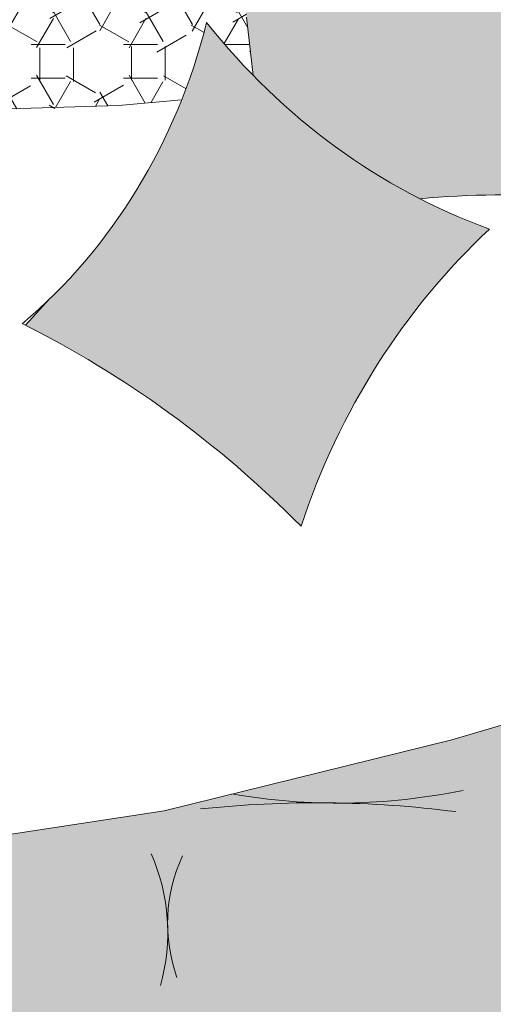
# Model space of a CAD drawing. Units: inches. Extents: x 1994 to 3075, y 3517 to 3950.
# Tile 43 of 58: x 1994.65094 to 1994.66748, y 3553.72103 to 3553.75542. Entities that reach past the tile are written whole.
import ezdxf

# ---------------------------------------------------------------- set-up
doc = ezdxf.new("R2010")
doc.units = ezdxf.units.IN
doc.layers.add('A-FURN-REFR', color=8, linetype='Continuous', lineweight=13)
doc.layers.add('A-FURN-REFR-PATT', color=8, linetype='Continuous', lineweight=13)

msp = doc.modelspace()

# ---------------------------------------------------------------- hatches: boundary and pattern name
at = {"layer": 'A-FURN-REFR-PATT'}
h = msp.add_hatch(dxfattribs=at)
h.set_pattern_fill('ESA_QT1', color=256, scale=0.001181, style=0, pattern_type=2)
h.set_pattern_definition([(0, (2000.7131367, 3549.95567), (0.0016133858, 0.0027944882), [0.0011811024, -0.0020457874]), (0, (2000.7131367, 3549.956851), (0.0016133858, 0.0027944882), [0.0011811024, -0.0020457874]), (60, (2000.7147507, 3549.9540566), (-0.0016134048, 0.0027944772), [0.0011811024, -0.0020457874]), (60, (2000.7137272, 3549.9546472), (-0.0016134048, 0.0027944772), [0.0011811024, -0.0020457874]), (120, (2000.7159311, 3549.9540566), (-0.0032267907, -1.1e-08), [0.0011811024, -0.0020457874]), (120, (2000.716954, 3549.9546472), (-0.0032267907, -1.1e-08), [0.0011811024, -0.0020457874]), (90, (2000.7131367, 3549.95567), (-0.00161338583, 0.0027944882), [0.0011811024, -0.0044079921]), (90, (2000.7143178, 3549.95567), (-0.00161338583, 0.0027944882), [0.0011811024, -0.0044079921]), (30, (2000.7159311, 3549.9540566), (0.00161340485, 0.0027944772), [0.0011811024, -0.0044079921]), (150, (2000.71475, 3549.9540566), (-0.00322679068, 1.1e-08), [0.0011811024, -0.0044079921]), (30, (2000.7153406, 3549.9550795), (0.00161340485, 0.0027944772), [0.0011811024, -0.0044079921]), (150, (2000.7153406, 3549.9550795), (-0.00322679068, 1.1e-08), [0.0011811024, -0.0044079921])])
edge = h.paths.add_edge_path()
edge.add_ellipse((1994.640876, 3553.752584), major_axis=(0, 0.019971), ratio=0.910403, start_angle=279.2385, end_angle=295.7126)
edge.add_ellipse((1994.661382, 3553.784799), major_axis=(0, 0.024564), ratio=0.910403, start_angle=170.9484, end_angle=180.8636)
edge.add_line((1994.661753, 3553.760238), (1994.660448, 3553.761168))
edge.add_line((1994.660448, 3553.761168), (1994.657839, 3553.762473))
edge.add_line((1994.657839, 3553.762473), (1994.656621, 3553.763504))
edge.add_line((1994.656621, 3553.763504), (1994.655861, 3553.763272))
edge.add_line((1994.655861, 3553.763272), (1994.655293, 3553.763476))
edge.add_line((1994.655293, 3553.763476), (1994.655493, 3553.762522))
edge.add_line((1994.655493, 3553.762522), (1994.655292, 3553.760584))
edge.add_line((1994.655292, 3553.760584), (1994.655292, 3553.760424))
edge.add_line((1994.655292, 3553.760424), (1994.655994, 3553.759788))
edge.add_line((1994.655994, 3553.759788), (1994.656079, 3553.758256))
edge.add_line((1994.656079, 3553.758256), (1994.654831, 3553.75802))
edge.add_line((1994.654831, 3553.75802), (1994.653607, 3553.75863))
edge.add_line((1994.653607, 3553.75863), (1994.651194, 3553.757931))
edge.add_line((1994.651194, 3553.757931), (1994.647697, 3553.757851))
edge.add_line((1994.647697, 3553.757851), (1994.645839, 3553.758008))
edge.add_line((1994.645839, 3553.758008), (1994.644836, 3553.757661))
edge.add_line((1994.644836, 3553.757661), (1994.64177, 3553.757379))
edge.add_line((1994.64177, 3553.757379), (1994.63952, 3553.757537))
edge.add_line((1994.63952, 3553.757537), (1994.636664, 3553.757269))
edge.add_line((1994.636664, 3553.757269), (1994.635142, 3553.757511))
edge.add_line((1994.635142, 3553.757511), (1994.634583, 3553.7569))
edge.add_line((1994.634583, 3553.7569), (1994.633061, 3553.756568))
edge.add_line((1994.633061, 3553.756568), (1994.631936, 3553.756647))
edge.add_line((1994.631936, 3553.756647), (1994.631946, 3553.757723))
edge.add_line((1994.631946, 3553.757723), (1994.632293, 3553.759053))
edge.add_line((1994.632293, 3553.759053), (1994.631942, 3553.760336))
edge.add_line((1994.631942, 3553.760336), (1994.631857, 3553.761868))
edge.add_line((1994.631857, 3553.761868), (1994.63213, 3553.76327))
edge.add_line((1994.63213, 3553.76327), (1994.632168, 3553.765117))
edge.add_line((1994.632168, 3553.765117), (1994.631874, 3553.766635))
edge.add_line((1994.631874, 3553.766635), (1994.632212, 3553.768118))
edge.add_line((1994.632212, 3553.768118), (1994.631521, 3553.769225))
edge.add_line((1994.631521, 3553.769225), (1994.631256, 3553.770206))
edge.add_line((1994.631256, 3553.770206), (1994.631719, 3553.770698))
edge.add_line((1994.631719, 3553.770698), (1994.632688, 3553.770917))
edge.add_line((1994.632688, 3553.770917), (1994.633747, 3553.770757))
edge.add_line((1994.633747, 3553.770757), (1994.63499, 3553.77107))
edge.add_line((1994.63499, 3553.77107), (1994.637864, 3553.771031))
edge.add_line((1994.637864, 3553.771031), (1994.638857, 3553.770678))
edge.add_line((1994.638857, 3553.770678), (1994.641165, 3553.770867))
edge.add_line((1994.641165, 3553.770867), (1994.645224, 3553.770907))
edge.add_line((1994.645224, 3553.770907), (1994.645865, 3553.770719))
edge.add_line((1994.645865, 3553.770719), (1994.647785, 3553.771462))
edge.add_line((1994.647785, 3553.771462), (1994.650215, 3553.771855))
edge.add_line((1994.650215, 3553.771855), (1994.65289, 3553.771785))
edge.add_line((1994.65289, 3553.771785), (1994.653416, 3553.772222))
edge.add_line((1994.653416, 3553.772222), (1994.654716, 3553.77277))
edge.add_line((1994.654716, 3553.77277), (1994.655776, 3553.77261))
edge.add_line((1994.655776, 3553.77261), (1994.655708, 3553.771299))
edge.add_line((1994.655708, 3553.771299), (1994.655135, 3553.770261))
edge.add_line((1994.655135, 3553.770261), (1994.655243, 3553.769577))
edge.add_line((1994.655243, 3553.769577), (1994.655057, 3553.767873))
edge.add_line((1994.655057, 3553.767873), (1994.655113, 3553.767736))
edge.add_line((1994.655113, 3553.767736), (1994.655702, 3553.76907))
edge.add_line((1994.655702, 3553.76907), (1994.656565, 3553.770145))
edge.add_line((1994.656565, 3553.770145), (1994.657423, 3553.771734))
edge.add_line((1994.657423, 3553.771734), (1994.657844, 3553.773215))
edge.add_line((1994.657844, 3553.773215), (1994.658028, 3553.77343))
edge.add_line((1994.658028, 3553.77343), (1994.632244, 3553.77343))
edge.add_ellipse((1994.632244, 3553.771319), major_axis=(0, 0.002111), ratio=0.910403, start_angle=0, end_angle=90)
edge.add_line((1994.630322, 3553.771319), (1994.630322, 3553.749441))
edge.add_line((1994.630322, 3553.749441), (1994.637709, 3553.750433))
edge.add_line((1994.637709, 3553.750433), (1994.645849, 3553.752088))
edge.add_line((1994.645849, 3553.752088), (1994.649254, 3553.75227))
edge.add_line((1994.649254, 3553.75227), (1994.654398, 3553.752423))
edge.add_line((1994.654398, 3553.752423), (1994.656593, 3553.752621))
edge.add_ellipse((1994.639937, 3553.760628), major_axis=(0, 0.019971), ratio=0.910403, start_angle=244.323, end_angle=253.1594)
edge.add_ellipse((1994.674344, 3553.771437), major_axis=(0, 0.024564), ratio=0.910403, start_angle=133.6721, end_angle=139.6806)
edge.add_line((1994.659095, 3553.753469), (1994.658861, 3553.755509))
edge = h.paths.add_edge_path()
edge.add_ellipse((1994.680284, 3553.771319), major_axis=(0, 0.002111), ratio=0.910403, start_angle=270, end_angle=360)
edge.add_line((1994.680284, 3553.77343), (1994.665356, 3553.77343))
edge.add_line((1994.665356, 3553.77343), (1994.665734, 3553.77298))
edge.add_line((1994.665734, 3553.77298), (1994.66783, 3553.771902))
edge.add_line((1994.66783, 3553.771902), (1994.671387, 3553.769751))
edge.add_line((1994.671387, 3553.769751), (1994.671861, 3553.769242))
edge.add_line((1994.671861, 3553.769242), (1994.673866, 3553.768856))
edge.add_line((1994.673866, 3553.768856), (1994.676159, 3553.76789))
edge.add_line((1994.676159, 3553.76789), (1994.67846, 3553.766389))
edge.add_line((1994.67846, 3553.766389), (1994.679113, 3553.766487))
edge.add_line((1994.679113, 3553.766487), (1994.680491, 3553.766264))
edge.add_line((1994.680491, 3553.766264), (1994.681343, 3553.765554))
edge.add_line((1994.681343, 3553.765554), (1994.680699, 3553.764448))
edge.add_line((1994.680699, 3553.764448), (1994.679737, 3553.763852))
edge.add_line((1994.679737, 3553.763852), (1994.679525, 3553.763197))
edge.add_line((1994.679525, 3553.763197), (1994.678603, 3553.761813))
edge.add_line((1994.678603, 3553.761813), (1994.678548, 3553.76116))
edge.add_line((1994.678548, 3553.76116), (1994.678066, 3553.759541))
edge.add_line((1994.678066, 3553.759541), (1994.676936, 3553.75803))
edge.add_line((1994.676936, 3553.75803), (1994.676848, 3553.757857))
edge.add_line((1994.676848, 3553.757857), (1994.676595, 3553.756914))
edge.add_line((1994.676595, 3553.756914), (1994.675477, 3553.755213))
edge.add_line((1994.675477, 3553.755213), (1994.675812, 3553.754261))
edge.add_line((1994.675812, 3553.754261), (1994.675202, 3553.75288))
edge.add_line((1994.675202, 3553.75288), (1994.674009, 3553.753346))
edge.add_line((1994.674009, 3553.753346), (1994.673214, 3553.754537))
edge.add_line((1994.673214, 3553.754537), (1994.670799, 3553.755226))
edge.add_line((1994.670799, 3553.755226), (1994.66897, 3553.756302))
edge.add_ellipse((1994.691382, 3553.757287), major_axis=(0, 0.024638), ratio=0.910403, start_angle=92.5166, end_angle=102.9728)
edge.add_line((1994.66943, 3553.75223), (1994.673814, 3553.75171))
edge.add_line((1994.673814, 3553.75171), (1994.677653, 3553.751587))
edge.add_line((1994.677653, 3553.751587), (1994.682205, 3553.751587))
edge.add_line((1994.682205, 3553.751587), (1994.682205, 3553.755102))
edge.add_line((1994.682205, 3553.755102), (1994.682205, 3553.771319))
h = msp.add_hatch(color=256, dxfattribs=at)
h.set_gradient(color1=(223, 184, 155), color2=(248, 239, 232), one_color=1, tint=0.94, name='SPHERICAL')
edge = h.paths.add_edge_path()
edge.add_ellipse((1994.691382, 3553.757287), major_axis=(0, 0.024638), ratio=0.910403, start_angle=92.5166, end_angle=102.9728, ccw=False)
edge.add_ellipse((1994.691382, 3553.757287), major_axis=(0, 0.024638), ratio=0.910403, start_angle=78.3263, end_angle=92.5166, ccw=False)
edge.add_ellipse((1994.661382, 3553.784799), major_axis=(0, 0.024564), ratio=0.910403, start_angle=180.8636, end_angle=199.1151, ccw=False)
edge.add_ellipse((1994.661382, 3553.784799), major_axis=(0, 0.024564), ratio=0.910403, start_angle=170.9484, end_angle=180.8636, ccw=False)
edge.add_ellipse((1994.640876, 3553.752584), major_axis=(0, 0.019971), ratio=0.910403, start_angle=279.2385, end_angle=295.7126, ccw=False)
edge.add_line((1994.658861, 3553.755509), (1994.659095, 3553.753469))
edge.add_ellipse((1994.674344, 3553.771437), major_axis=(0, 0.024564), ratio=0.910403, start_angle=139.6806, end_angle=157.0382)
edge.add_ellipse((1994.66794, 3553.708563), major_axis=(0, 0.04074), ratio=0.910403, start_angle=356.8603, end_angle=364.2706, ccw=False)
edge.add_line((1994.670171, 3553.749229), (1994.670182, 3553.749241))
edge.add_ellipse((1994.691382, 3553.757287), major_axis=(0, 0.024638), ratio=0.910403, start_angle=102.9728, end_angle=110.7835, ccw=False)
h = msp.add_hatch(color=256, dxfattribs=at)
h.set_gradient(color1=(216, 161, 105), color2=(246, 232, 219), one_color=1, tint=0.91, name='SPHERICAL')
edge = h.paths.add_edge_path()
edge.add_ellipse((1994.674344, 3553.771437), major_axis=(0, 0.024564), ratio=0.910403, start_angle=157.0382, end_angle=163.301, ccw=False)
edge.add_ellipse((1994.674344, 3553.771437), major_axis=(0, 0.024564), ratio=0.910403, start_angle=139.6806, end_angle=157.0382, ccw=False)
edge.add_ellipse((1994.674344, 3553.771437), major_axis=(0, 0.024564), ratio=0.910403, start_angle=133.6721, end_angle=139.6806, ccw=False)
edge.add_ellipse((1994.639937, 3553.760628), major_axis=(0, 0.019971), ratio=0.910403, start_angle=244.323, end_angle=253.1594, ccw=False)
edge.add_ellipse((1994.639937, 3553.760628), major_axis=(0, 0.019971), ratio=0.910403, start_angle=218.8801, end_angle=244.323, ccw=False)
edge.add_line((1994.651992, 3553.745678), (1994.651144, 3553.744747))
edge.add_ellipse((1994.635682, 3553.707716), major_axis=(0, 0.04074), ratio=0.910403, start_angle=320.1141, end_angle=337.338, ccw=False)
edge.add_ellipse((1994.681843, 3553.729307), major_axis=(0, 0.024638), ratio=0.910403, start_angle=397.6398, end_angle=428.2251, ccw=False)
h = msp.add_hatch(color=256, dxfattribs=at)
h.set_gradient(color1=(238, 215, 180), color2=(243, 226, 201), one_color=1, tint=0.87)
edge = h.paths.add_edge_path()
edge.add_line((1994.681542, 3553.709525), (1994.682048, 3553.709217))
edge.add_line((1994.682048, 3553.709217), (1994.682631, 3553.708815))
edge.add_line((1994.682631, 3553.708815), (1994.682631, 3553.708383))
edge.add_line((1994.682631, 3553.708383), (1994.682498, 3553.704652))
edge.add_line((1994.682498, 3553.704652), (1994.682631, 3553.701474))
edge.add_line((1994.682631, 3553.701474), (1994.682631, 3553.700426))
edge.add_line((1994.682631, 3553.700426), (1994.682104, 3553.700396))
edge.add_line((1994.682104, 3553.700396), (1994.681598, 3553.699902))
edge.add_line((1994.681598, 3553.699902), (1994.681992, 3553.699717))
edge.add_line((1994.681992, 3553.699717), (1994.682631, 3553.699439))
edge.add_line((1994.682631, 3553.699439), (1994.682631, 3553.695334))
edge.add_ellipse((1994.680709, 3553.695334), major_axis=(0, 0.002111), ratio=0.910403, start_angle=180, end_angle=270, ccw=False)
edge.add_line((1994.680709, 3553.693223), (1994.680522, 3553.693223))
edge.add_line((1994.680522, 3553.693223), (1994.680314, 3553.694))
edge.add_ellipse((1994.68491, 3553.694998), major_axis=(0, 0.005146), ratio=0.910403, start_angle=92.3431, end_angle=102.2543, ccw=False)
edge.add_ellipse((1994.674568, 3553.694683), major_axis=(0, 0.006219), ratio=0.910403, start_angle=-88.7485, end_angle=-87.76)
edge.add_ellipse((1994.68491, 3553.694998), major_axis=(0, 0.005146), ratio=0.910403, start_angle=91.1484, end_angle=92.3431)
edge.add_ellipse((1994.674568, 3553.694683), major_axis=(0, 0.006219), ratio=0.910403, start_angle=262.8125, end_angle=271.2515, ccw=False)
edge.add_line((1994.680193, 3553.693973), (1994.679278, 3553.693223))
edge.add_line((1994.679278, 3553.693223), (1994.678042, 3553.693223))
edge.add_line((1994.678042, 3553.693223), (1994.673955, 3553.693055))
edge.add_line((1994.673955, 3553.693055), (1994.669892, 3553.693223))
edge.add_line((1994.669892, 3553.693223), (1994.669387, 3553.693223))
edge.add_line((1994.669387, 3553.693223), (1994.668536, 3553.693813))
edge.add_ellipse((1994.673095, 3553.694999), major_axis=(0, 0.005146), ratio=0.910403, start_angle=92.3431, end_angle=104.5922, ccw=False)
edge.add_ellipse((1994.662753, 3553.694684), major_axis=(0, 0.006219), ratio=0.910403, start_angle=-88.7485, end_angle=-87.76)
edge.add_ellipse((1994.673095, 3553.694999), major_axis=(0, 0.005146), ratio=0.910403, start_angle=91.1484, end_angle=92.3431)
edge.add_ellipse((1994.662753, 3553.694684), major_axis=(0, 0.006219), ratio=0.910403, start_angle=260.6759, end_angle=271.2515, ccw=False)
edge.add_line((1994.668352, 3553.693765), (1994.66822, 3553.693223))
edge.add_line((1994.66822, 3553.693223), (1994.666295, 3553.693223))
edge.add_line((1994.666295, 3553.693223), (1994.664702, 3553.693298))
edge.add_line((1994.664702, 3553.693298), (1994.660712, 3553.693051))
edge.add_line((1994.660712, 3553.693051), (1994.65764, 3553.693223))
edge.add_line((1994.65764, 3553.693223), (1994.656797, 3553.693223))
edge.add_line((1994.656797, 3553.693223), (1994.656116, 3553.693819))
edge.add_ellipse((1994.660616, 3553.695249), major_axis=(0, 0.005146), ratio=0.910403, start_angle=92.3431, end_angle=107.6246, ccw=False)
edge.add_ellipse((1994.650274, 3553.694934), major_axis=(0, 0.006219), ratio=0.910403, start_angle=-88.7485, end_angle=-87.76)
edge.add_ellipse((1994.660616, 3553.695249), major_axis=(0, 0.005146), ratio=0.910403, start_angle=91.1484, end_angle=92.3431)
edge.add_ellipse((1994.650274, 3553.694934), major_axis=(0, 0.006219), ratio=0.910403, start_angle=257.752, end_angle=271.2515, ccw=False)
edge.add_line((1994.655829, 3553.693728), (1994.654998, 3553.693223))
edge.add_line((1994.654998, 3553.693223), (1994.649752, 3553.692989))
edge.add_line((1994.649752, 3553.692989), (1994.644994, 3553.693223))
edge.add_line((1994.644994, 3553.693223), (1994.643952, 3553.693223))
edge.add_ellipse((1994.651853, 3553.695067), major_axis=(0, 0.008872), ratio=0.910403, start_angle=89.8354, end_angle=103.1369, ccw=False)
edge.add_ellipse((1994.638929, 3553.695405), major_axis=(0, 0.005332), ratio=0.910403, start_angle=266.2788, end_angle=270.7223)
edge.add_ellipse((1994.651853, 3553.695067), major_axis=(0, 0.008872), ratio=0.910403, start_angle=87.1651, end_angle=89.8354)
edge.add_ellipse((1994.638929, 3553.695405), major_axis=(0, 0.005332), ratio=0.910403, start_angle=243.7698, end_angle=266.2788, ccw=False)
edge.add_line((1994.643359, 3553.693223), (1994.642545, 3553.693223))
edge.add_line((1994.642545, 3553.693223), (1994.641153, 3553.693113))
edge.add_line((1994.641153, 3553.693113), (1994.636432, 3553.693359))
edge.add_line((1994.636432, 3553.693359), (1994.633777, 3553.693223))
edge.add_line((1994.633777, 3553.693223), (1994.63245, 3553.693223))
edge.add_line((1994.63245, 3553.693223), (1994.632375, 3553.693314))
edge.add_ellipse((1994.640193, 3553.695548), major_axis=(0, 0.008872), ratio=0.910403, start_angle=89.8354, end_angle=105.9456, ccw=False)
edge.add_ellipse((1994.627269, 3553.695886), major_axis=(0, 0.005332), ratio=0.910403, start_angle=266.2788, end_angle=270.7223)
edge.add_ellipse((1994.640193, 3553.695548), major_axis=(0, 0.008872), ratio=0.910403, start_angle=87.1651, end_angle=89.8354)
edge.add_ellipse((1994.627269, 3553.695886), major_axis=(0, 0.005332), ratio=0.910403, start_angle=237.8324, end_angle=266.2788, ccw=False)
edge.add_ellipse((1994.6317, 3553.695334), major_axis=(0, 0.002111), ratio=0.910403, start_angle=90, end_angle=174.0631, ccw=False)
edge.add_line((1994.629778, 3553.695334), (1994.629737, 3553.696763))
edge.add_line((1994.629737, 3553.696763), (1994.629778, 3553.698454))
edge.add_line((1994.629778, 3553.698454), (1994.629778, 3553.699441))
edge.add_line((1994.629778, 3553.699441), (1994.629962, 3553.700094))
edge.add_line((1994.629962, 3553.700094), (1994.630637, 3553.700403))
edge.add_line((1994.630637, 3553.700403), (1994.630075, 3553.700834))
edge.add_line((1994.630075, 3553.700834), (1994.629778, 3553.701292))
edge.add_line((1994.629778, 3553.701292), (1994.629778, 3553.702155))
edge.add_line((1994.629778, 3553.702155), (1994.630018, 3553.703363))
edge.add_line((1994.630018, 3553.703363), (1994.630018, 3553.706016))
edge.add_line((1994.630018, 3553.706016), (1994.629778, 3553.708015))
edge.add_line((1994.629778, 3553.708015), (1994.629778, 3553.70894))
edge.add_line((1994.629778, 3553.70894), (1994.630187, 3553.709347))
edge.add_line((1994.630187, 3553.709347), (1994.630918, 3553.70947))
edge.add_line((1994.630918, 3553.70947), (1994.630299, 3553.709902))
edge.add_line((1994.630299, 3553.709902), (1994.629778, 3553.710112))
edge.add_line((1994.629778, 3553.710112), (1994.629778, 3553.712086))
edge.add_line((1994.629778, 3553.712086), (1994.629962, 3553.713788))
edge.add_line((1994.629962, 3553.713788), (1994.629778, 3553.716158))
edge.add_line((1994.629778, 3553.716158), (1994.629778, 3553.718502))
edge.add_line((1994.629778, 3553.718502), (1994.630187, 3553.718908))
edge.add_line((1994.630187, 3553.718908), (1994.629778, 3553.719365))
edge.add_line((1994.629778, 3553.719365), (1994.629778, 3553.72115))
edge.add_line((1994.629778, 3553.72115), (1994.630322, 3553.72115))
edge.add_line((1994.630322, 3553.72115), (1994.634865, 3553.721849))
edge.add_line((1994.634865, 3553.721849), (1994.639494, 3553.724204))
edge.add_line((1994.639494, 3553.724204), (1994.643653, 3553.725608))
edge.add_ellipse((1994.63891, 3553.72447), major_axis=(0, 0.005332), ratio=0.910403, start_angle=270.7223, end_angle=283.4893, ccw=False)
edge.add_ellipse((1994.651833, 3553.724132), major_axis=(0, 0.008872), ratio=0.910403, start_angle=87.1651, end_angle=89.8354)
edge.add_ellipse((1994.63891, 3553.72447), major_axis=(0, 0.005332), ratio=0.910403, start_angle=266.2788, end_angle=270.7223)
edge.add_ellipse((1994.651833, 3553.724132), major_axis=(0, 0.008872), ratio=0.910403, start_angle=438.9501, end_angle=447.1651, ccw=False)
edge.add_line((1994.643881, 3553.725685), (1994.643897, 3553.72569))
edge.add_line((1994.643897, 3553.72569), (1994.649542, 3553.726806))
edge.add_line((1994.649542, 3553.726806), (1994.655977, 3553.727797))
edge.add_line((1994.655977, 3553.727797), (1994.658348, 3553.728382))
edge.add_ellipse((1994.662052, 3553.754177), major_axis=(0, 0.026115), ratio=0.910403, start_angle=171.8281, end_angle=180.2609)
edge.add_ellipse((1994.661314, 3553.682223), major_axis=(0, 0.04585), ratio=0.910403, start_angle=-1.0711, end_angle=-0.1044)
edge.add_ellipse((1994.662052, 3553.754177), major_axis=(0, 0.026115), ratio=0.910403, start_angle=171.8281, end_angle=178.5636, ccw=False)
edge.add_line((1994.658348, 3553.728382), (1994.666025, 3553.730275))
edge.add_line((1994.666025, 3553.730275), (1994.67483, 3553.732877))
edge.add_line((1994.67483, 3553.732877), (1994.680219, 3553.734687))
edge.add_ellipse((1994.675489, 3553.733489), major_axis=(0, 0.005332), ratio=0.910403, start_angle=270.7223, end_angle=284.2178, ccw=False)
edge.add_ellipse((1994.688412, 3553.73315), major_axis=(0, 0.008872), ratio=0.910403, start_angle=87.1651, end_angle=89.8354)
edge.add_ellipse((1994.675489, 3553.733489), major_axis=(0, 0.005332), ratio=0.910403, start_angle=266.2788, end_angle=270.7223)
edge.add_ellipse((1994.688412, 3553.73315), major_axis=(0, 0.008872), ratio=0.910403, start_angle=438.5005, end_angle=447.1651, ccw=False)
edge.add_line((1994.68047, 3553.734766), (1994.682205, 3553.735263))
edge.add_line((1994.682205, 3553.735263), (1994.682631, 3553.735263))
edge.add_line((1994.682631, 3553.735263), (1994.682631, 3553.734609))
edge.add_line((1994.682631, 3553.734609), (1994.682783, 3553.733623))
edge.add_line((1994.682783, 3553.733623), (1994.682631, 3553.730537))
edge.add_line((1994.682631, 3553.730537), (1994.682631, 3553.728749))
edge.add_line((1994.682631, 3553.728749), (1994.682334, 3553.728195))
edge.add_line((1994.682334, 3553.728195), (1994.681547, 3553.727824))
edge.add_line((1994.681547, 3553.727824), (1994.682053, 3553.727639))
edge.add_line((1994.682053, 3553.727639), (1994.682631, 3553.72733))
edge.add_line((1994.682631, 3553.72733), (1994.682631, 3553.725726))
edge.add_line((1994.682631, 3553.725726), (1994.682727, 3553.724308))
edge.add_line((1994.682727, 3553.724308), (1994.682631, 3553.721716))
edge.add_line((1994.682631, 3553.721716), (1994.682631, 3553.720165))
edge.add_line((1994.682631, 3553.720165), (1994.682329, 3553.719086))
edge.add_line((1994.682329, 3553.719086), (1994.681823, 3553.718654))
edge.add_line((1994.681823, 3553.718654), (1994.682329, 3553.718531))
edge.add_line((1994.682329, 3553.718531), (1994.682722, 3553.718346))
edge.add_line((1994.682722, 3553.718346), (1994.68261, 3553.715693))
edge.add_line((1994.68261, 3553.715693), (1994.682631, 3553.711159))
edge.add_line((1994.682631, 3553.711159), (1994.682631, 3553.710327))
edge.add_line((1994.682631, 3553.710327), (1994.682217, 3553.70971))
edge.add_line((1994.682217, 3553.70971), (1994.681542, 3553.709525))
edge = h.paths.add_edge_path(flags=16)
edge.add_ellipse((1994.674017, 3553.663488), major_axis=(0, 0.04585), ratio=0.910403, start_angle=-1.0711, end_angle=-0.1044)
edge.add_ellipse((1994.674755, 3553.735442), major_axis=(0, 0.026115), ratio=0.910403, start_angle=178.5636, end_angle=180.2609)
h.paths.add_polyline_path([(1994.668419, 3553.710039), (1994.668385, 3553.710026), (1994.668404, 3553.710013)], flags=16)
edge = h.paths.add_edge_path(flags=16)
edge.add_ellipse((1994.663397, 3553.714852), major_axis=(0, 0.005332), ratio=0.910403, start_angle=266.2788, end_angle=270.7223)
edge.add_ellipse((1994.67632, 3553.714514), major_axis=(0, 0.008872), ratio=0.910403, start_angle=87.1651, end_angle=89.8354)
edge = h.paths.add_edge_path(flags=16)
edge.add_ellipse((1994.662753, 3553.703926), major_axis=(0, 0.006219), ratio=0.910403, start_angle=-88.7485, end_angle=-87.76)
edge.add_ellipse((1994.673095, 3553.704241), major_axis=(0, 0.005146), ratio=0.910403, start_angle=91.1484, end_angle=92.3431)
h.paths.add_polyline_path([(1994.680357, 3553.710026), (1994.680376, 3553.710013), (1994.680391, 3553.710039)], flags=16)
edge = h.paths.add_edge_path(flags=16)
edge.add_ellipse((1994.684791, 3553.713857), major_axis=(0, 0.005146), ratio=0.910403, start_angle=91.1484, end_angle=92.3431)
edge.add_ellipse((1994.67445, 3553.713542), major_axis=(0, 0.006219), ratio=0.910403, start_angle=-88.7485, end_angle=-87.76)
h.paths.add_polyline_path([(1994.668404, 3553.719229), (1994.668419, 3553.719256), (1994.668385, 3553.719242)], flags=16)
edge = h.paths.add_edge_path(flags=16)
edge.add_ellipse((1994.68491, 3553.704625), major_axis=(0, 0.005146), ratio=0.910403, start_angle=91.1484, end_angle=92.3431)
edge.add_ellipse((1994.674568, 3553.70431), major_axis=(0, 0.006219), ratio=0.910403, start_angle=-88.7485, end_angle=-87.76)
edge = h.paths.add_edge_path(flags=16)
edge.add_ellipse((1994.662353, 3553.744655), major_axis=(0, 0.026115), ratio=0.910403, start_angle=178.5636, end_angle=180.2609)
edge.add_ellipse((1994.661615, 3553.6727), major_axis=(0, 0.04585), ratio=0.910403, start_angle=-1.0711, end_angle=-0.1044)
edge = h.paths.add_edge_path(flags=16)
edge.add_ellipse((1994.662621, 3553.722979), major_axis=(0, 0.006219), ratio=0.910403, start_angle=-88.7485, end_angle=-87.76)
edge.add_ellipse((1994.672963, 3553.723294), major_axis=(0, 0.005146), ratio=0.910403, start_angle=91.1484, end_angle=92.3431)
h.paths.add_polyline_path([(1994.68017, 3553.719242), (1994.680189, 3553.719229), (1994.680204, 3553.719256)], flags=16)
h.paths.add_polyline_path([(1994.668419, 3553.70036), (1994.668385, 3553.700347), (1994.668404, 3553.700334)], flags=16)
edge = h.paths.add_edge_path(flags=16)
edge.add_ellipse((1994.673942, 3553.654177), major_axis=(0, 0.04585), ratio=0.910403, start_angle=-1.0711, end_angle=-0.1044)
edge.add_ellipse((1994.67468, 3553.726132), major_axis=(0, 0.026115), ratio=0.910403, start_angle=178.5636, end_angle=180.2609)
edge = h.paths.add_edge_path(flags=16)
edge.add_ellipse((1994.685026, 3553.723294), major_axis=(0, 0.005146), ratio=0.910403, start_angle=91.1484, end_angle=92.3431)
edge.add_ellipse((1994.674684, 3553.722979), major_axis=(0, 0.006219), ratio=0.910403, start_angle=-88.7485, end_angle=-87.76)
h.paths.add_polyline_path([(1994.680569, 3553.70036), (1994.680535, 3553.700347), (1994.680554, 3553.700334)], flags=16)
h.paths.add_polyline_path([(1994.656068, 3553.710085), (1994.656034, 3553.710071), (1994.656052, 3553.710058)], flags=16)
h.paths.add_polyline_path([(1994.668404, 3553.728426), (1994.668419, 3553.728453), (1994.668385, 3553.728439)], flags=16)
edge = h.paths.add_edge_path(flags=16)
edge.add_ellipse((1994.650317, 3553.713896), major_axis=(0, 0.006219), ratio=0.910403, start_angle=-88.7485, end_angle=-87.76)
edge.add_ellipse((1994.660659, 3553.714211), major_axis=(0, 0.005146), ratio=0.910403, start_angle=91.1484, end_angle=92.3431)
edge = h.paths.add_edge_path(flags=16)
edge.add_ellipse((1994.650274, 3553.70431), major_axis=(0, 0.006219), ratio=0.910403, start_angle=-88.7485, end_angle=-87.76)
edge.add_ellipse((1994.660616, 3553.704625), major_axis=(0, 0.005146), ratio=0.910403, start_angle=91.1484, end_angle=92.3431)
h.paths.add_polyline_path([(1994.68033, 3553.728439), (1994.680349, 3553.728426), (1994.680364, 3553.728453)], flags=16)
h.paths.add_polyline_path([(1994.656052, 3553.719229), (1994.656068, 3553.719256), (1994.656034, 3553.719242)], flags=16)
edge = h.paths.add_edge_path(flags=16)
edge.add_ellipse((1994.649569, 3553.663672), major_axis=(0, 0.04585), ratio=0.910403, start_angle=-1.0711, end_angle=-0.1044)
edge.add_ellipse((1994.650307, 3553.735627), major_axis=(0, 0.026115), ratio=0.910403, start_angle=178.5636, end_angle=180.2609)
h.paths.add_polyline_path([(1994.656068, 3553.700324), (1994.656034, 3553.70031), (1994.656052, 3553.700297)], flags=16)
edge = h.paths.add_edge_path(flags=16)
edge.add_ellipse((1994.650446, 3553.723545), major_axis=(0, 0.006219), ratio=0.910403, start_angle=-88.7485, end_angle=-87.76)
edge.add_ellipse((1994.660788, 3553.72386), major_axis=(0, 0.005146), ratio=0.910403, start_angle=91.1484, end_angle=92.3431)
edge = h.paths.add_edge_path(flags=16)
edge.add_ellipse((1994.64966, 3553.654177), major_axis=(0, 0.04585), ratio=0.910403, start_angle=-1.0711, end_angle=-0.1044)
edge.add_ellipse((1994.650398, 3553.726132), major_axis=(0, 0.026115), ratio=0.910403, start_angle=178.5636, end_angle=180.2609)
h.paths.add_polyline_path([(1994.643774, 3553.710039), (1994.64374, 3553.710026), (1994.643759, 3553.710013)], flags=16)
edge = h.paths.add_edge_path(flags=16)
edge.add_ellipse((1994.638006, 3553.713542), major_axis=(0, 0.006219), ratio=0.910403, start_angle=-88.7485, end_angle=-87.76)
edge.add_ellipse((1994.648347, 3553.713857), major_axis=(0, 0.005146), ratio=0.910403, start_angle=91.1484, end_angle=92.3431)
edge = h.paths.add_edge_path(flags=16)
edge.add_ellipse((1994.638929, 3553.705498), major_axis=(0, 0.005332), ratio=0.910403, start_angle=266.2788, end_angle=270.7223)
edge.add_ellipse((1994.651853, 3553.705159), major_axis=(0, 0.008872), ratio=0.910403, start_angle=87.1651, end_angle=89.8354)
h.paths.add_polyline_path([(1994.643759, 3553.719229), (1994.643774, 3553.719256), (1994.64374, 3553.719242)], flags=16)
h.paths.add_polyline_path([(1994.643774, 3553.700752), (1994.64374, 3553.700739), (1994.643759, 3553.700726)], flags=16)
edge = h.paths.add_edge_path(flags=16)
edge.add_ellipse((1994.637078, 3553.672998), major_axis=(0, 0.04585), ratio=0.910403, start_angle=-1.0711, end_angle=-0.1044)
edge.add_ellipse((1994.637816, 3553.744953), major_axis=(0, 0.026115), ratio=0.910403, start_angle=178.5636, end_angle=180.2609)
edge = h.paths.add_edge_path(flags=16)
edge.add_ellipse((1994.637265, 3553.654177), major_axis=(0, 0.04585), ratio=0.910403, start_angle=-1.0711, end_angle=-0.1044)
edge.add_ellipse((1994.638003, 3553.726132), major_axis=(0, 0.026115), ratio=0.910403, start_angle=178.5636, end_angle=180.2609)
h.paths.add_polyline_path([(1994.632201, 3553.710039), (1994.632167, 3553.710026), (1994.632186, 3553.710013)], flags=16)
edge = h.paths.add_edge_path(flags=16)
edge.add_ellipse((1994.626452, 3553.713542), major_axis=(0, 0.006219), ratio=0.910403, start_angle=-88.7485, end_angle=-87.76)
edge.add_ellipse((1994.636794, 3553.713857), major_axis=(0, 0.005146), ratio=0.910403, start_angle=91.1484, end_angle=92.3431)
edge = h.paths.add_edge_path(flags=16)
edge.add_ellipse((1994.627269, 3553.705498), major_axis=(0, 0.005332), ratio=0.910403, start_angle=266.2788, end_angle=270.7223)
edge.add_ellipse((1994.640193, 3553.705159), major_axis=(0, 0.008872), ratio=0.910403, start_angle=87.1651, end_angle=89.8354)
h.paths.add_polyline_path([(1994.631818, 3553.719229), (1994.631834, 3553.719256), (1994.631799, 3553.719242)], flags=16)
h.paths.add_polyline_path([(1994.631864, 3553.700752), (1994.63183, 3553.700739), (1994.631849, 3553.700726)], flags=16)

# ---------------------------------------------------------------- linework, layer by layer
at = {"layer": 'A-FURN-REFR'}
for p, q in [((1994.658861, 3553.755509), (1994.659095, 3553.753469)), ((1994.649254, 3553.75227), (1994.654398, 3553.752423)), ((1994.654398, 3553.752423), (1994.656593, 3553.752621)), ((1994.651144, 3553.744747), (1994.651992, 3553.745678)), ((1994.666025, 3553.730275), (1994.67483, 3553.732877)), ((1994.655977, 3553.727797), (1994.666025, 3553.730275)), ((1994.649542, 3553.726806), (1994.655977, 3553.727797))]:
    msp.add_line(p, q, dxfattribs=at)
at = {"layer": 'A-FURN-REFR', "extrusion": (0, 0, -1)}
for centre, major_axis, start_param, end_param in [((1994.639937, 3553.760628), (0, 0.019971), 1.839693, 2.485458), ((1994.674344, 3553.771437), (0, 0.024564), 3.459906, 3.996881), ((1994.66794, 3553.708563), (0, 0.04074), -0.081839, 0.060591), ((1994.681843, 3553.729307), (0, 0.024638), -1.221994, -0.702813), ((1994.635682, 3553.707716), (0, 0.04074), 0.426594, 0.742647), ((1994.662052, 3553.754177), (0, 0.026115), 2.956807, 3.298037), ((1994.661314, 3553.682223), (0, 0.04585), -0.097463, 0.116495), ((1994.650446, 3553.723545), (0, 0.006219), 1.114213, 1.873711), ((1994.660788, 3553.72386), (0, 0.005146), 4.336804, 5.187972)]:
    msp.add_ellipse(centre, major_axis=major_axis, ratio=0.910403, start_param=start_param, end_param=end_param, dxfattribs=at)

doc.saveas('drawing.dxf')
